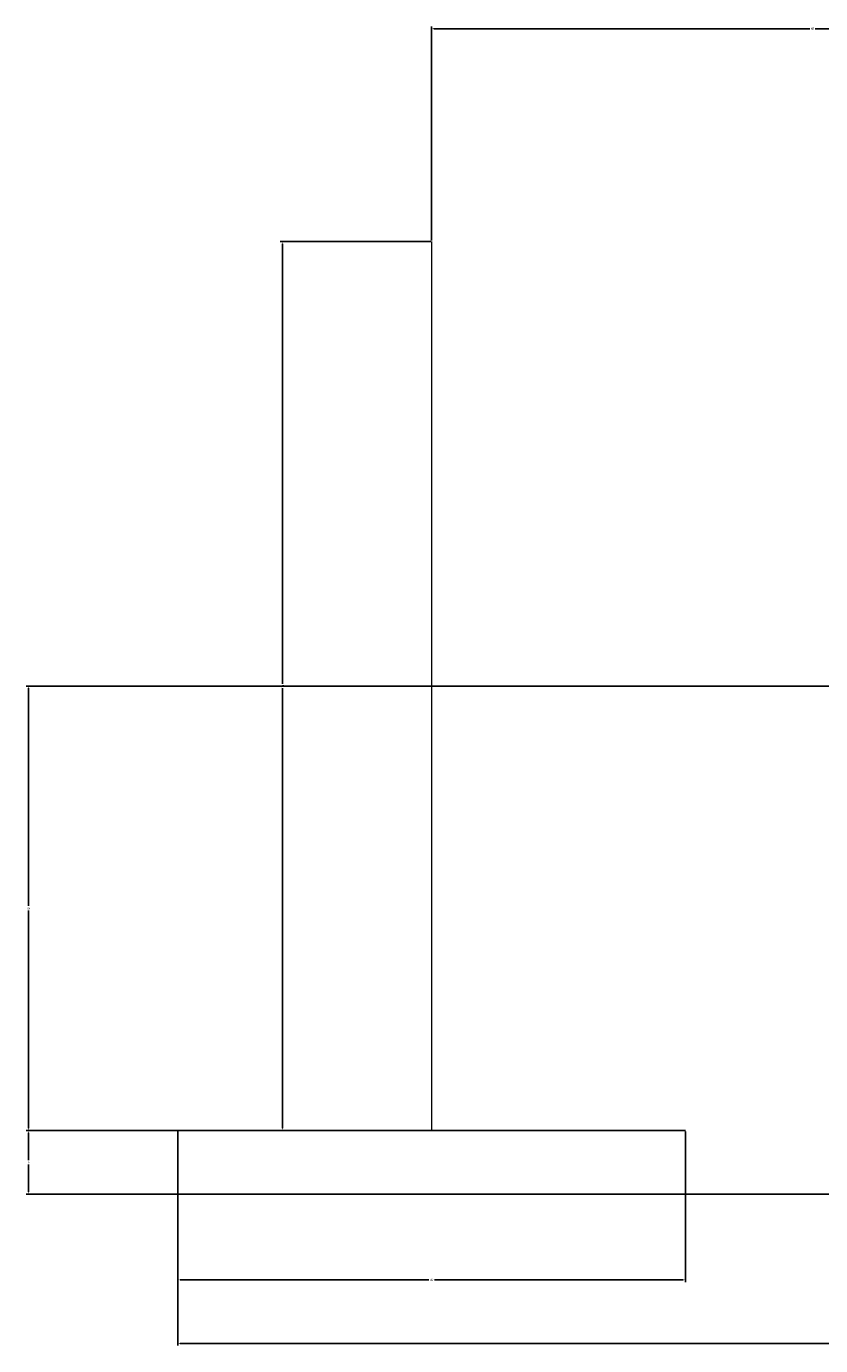
# Model space of a CAD drawing. Units: millimetres. Extents: x 3108 to 3332, y 1482 to 1586.
# Tile 1 of 5: x 3108 to 3171, y 1482 to 1586. Entities that reach past the tile are written whole.
import ezdxf

# ---------------------------------------------------------------- set-up
doc = ezdxf.new("R2010")
doc.units = ezdxf.units.MM
doc.layers.add('M-CONS', color=8, linetype='Continuous', lineweight=18)
doc.layers.add('M-DIMS', color=2, linetype='Continuous', lineweight=18)
doc.styles.get("Standard").update_dxf_attribs({"font": 'arial.ttf'})
doc.dimstyles.get("Standard").update_dxf_attribs({"dimtxt": 0.18, "dimasz": 0.18, "dimexe": 0.18, "dimexo": 0.0625, "dimgap": 0.09, "dimtad": 0, "dimtih": 1, "dimtoh": 1, "dimdec": 4, "dimzin": 0, "dimdsep": 46, "dimtxsty": 'Standard', "dimcen": 0.09, "dimadec": 0, "dimazin": 0, "dimtfac": 1, "dimtdec": 4, "dimtofl": 0, "dimtmove": 0, "dimatfit": 3, "dimfxl": 1, "dimtolj": 1, "dimtzin": 0, "dimarcsym": 0})

# ---------------------------------------------------------------- blocks, each defined once
blk = doc.blocks.new('*D1')
at = {"layer": 'Defpoints', "color": 0, "transparency": 16777216}
for p in [(3119.94, 1498.94), (3319.94, 1493.94), (3319.94, 1482.19)]:
    blk.add_point(p, dxfattribs=at)
at = {"layer": 'M-DIMS', "color": 0, "lineweight": -2, "transparency": 16777216}
for p, q in [((3119.94, 1498.88), (3119.94, 1482.01)), ((3319.94, 1493.88), (3319.94, 1482.01)), ((3120.12, 1482.19), (3219.65, 1482.19)), ((3319.76, 1482.19), (3220.23, 1482.19))]:
    blk.add_line(p, q, dxfattribs=at)
at = {"layer": 'M-DIMS', "color": 0, "transparency": 16777216}
for points in [[(3120.12, 1482.22), (3120.12, 1482.16), (3119.94, 1482.19)], [(3319.76, 1482.22), (3319.76, 1482.16), (3319.94, 1482.19)]]:
    blk.add_solid(points, dxfattribs=at)
at = {"layer": 'M-DIMS', "color": 0, "transparency": 16777216, "insert": (3219.94, 1482.19), "char_height": 0.18, "attachment_point": 5}
blk.add_mtext('\\A1;200', dxfattribs=at)
blk = doc.blocks.new('*D4')
at = {"layer": 'Defpoints', "color": 0, "transparency": 16777216}
for p in [(3119.94, 1498.94), (3159.94, 1498.94), (3119.94, 1487.19)]:
    blk.add_point(p, dxfattribs=at)
at = {"layer": 'M-DIMS', "color": 0, "lineweight": -2, "transparency": 16777216}
for p, q in [((3119.94, 1498.88), (3119.94, 1487.01)), ((3159.94, 1498.88), (3159.94, 1487.01)), ((3120.12, 1487.19), (3139.72, 1487.19)), ((3159.76, 1487.19), (3140.17, 1487.19))]:
    blk.add_line(p, q, dxfattribs=at)
at = {"layer": 'M-DIMS', "color": 0, "transparency": 16777216}
for points in [[(3120.12, 1487.22), (3120.12, 1487.16), (3119.94, 1487.19)], [(3159.76, 1487.22), (3159.76, 1487.16), (3159.94, 1487.19)]]:
    blk.add_solid(points, dxfattribs=at)
at = {"layer": 'M-DIMS', "color": 0, "transparency": 16777216, "insert": (3139.94, 1487.19), "char_height": 0.18, "attachment_point": 5}
blk.add_mtext('\\A1;40', dxfattribs=at)
blk = doc.blocks.new('*D5')
at = {"layer": 'Defpoints', "color": 0, "transparency": 16777216}
for p in [(3128.19, 1568.94), (3139.94, 1568.94), (3139.94, 1498.94)]:
    blk.add_point(p, dxfattribs=at)
at = {"layer": 'M-DIMS', "color": 0, "lineweight": -2, "transparency": 16777216}
for p, q in [((3139.88, 1568.94), (3128.01, 1568.94)), ((3128.19, 1568.76), (3128.19, 1534.12)), ((3128.19, 1499.12), (3128.19, 1533.76)), ((3139.88, 1498.94), (3128.01, 1498.94))]:
    blk.add_line(p, q, dxfattribs=at)
at = {"layer": 'M-DIMS', "color": 0, "transparency": 16777216}
for points in [[(3128.16, 1568.76), (3128.22, 1568.76), (3128.19, 1568.94)], [(3128.16, 1499.12), (3128.22, 1499.12), (3128.19, 1498.94)]]:
    blk.add_solid(points, dxfattribs=at)
at = {"layer": 'M-DIMS', "color": 0, "transparency": 16777216, "insert": (3128.19, 1533.94), "char_height": 0.18, "attachment_point": 5}
blk.add_mtext('\\A1;70', dxfattribs=at)
blk = doc.blocks.new('*D6')
at = {"layer": 'Defpoints', "color": 0, "transparency": 16777216}
for p in [(3199.94, 1585.69), (3139.94, 1568.94), (3199.94, 1533.94)]:
    blk.add_point(p, dxfattribs=at)
at = {"layer": 'M-DIMS', "color": 0, "lineweight": -2, "transparency": 16777216}
for p, q in [((3139.94, 1569.01), (3139.94, 1585.87)), ((3140.12, 1585.69), (3169.73, 1585.69)), ((3199.76, 1585.69), (3170.16, 1585.69)), ((3199.94, 1534.01), (3199.94, 1585.87))]:
    blk.add_line(p, q, dxfattribs=at)
at = {"layer": 'M-DIMS', "color": 0, "transparency": 16777216}
for points in [[(3140.12, 1585.72), (3140.12, 1585.66), (3139.94, 1585.69)], [(3199.76, 1585.72), (3199.76, 1585.66), (3199.94, 1585.69)]]:
    blk.add_solid(points, dxfattribs=at)
at = {"layer": 'M-DIMS', "color": 0, "transparency": 16777216, "insert": (3169.94, 1585.69), "char_height": 0.18, "attachment_point": 5}
blk.add_mtext('\\A1;60', dxfattribs=at)
blk = doc.blocks.new('*D9')
at = {"layer": 'Defpoints', "color": 0, "transparency": 16777216}
for p in [(3108.19, 1533.94), (3199.94, 1533.94), (3159.94, 1498.94)]:
    blk.add_point(p, dxfattribs=at)
at = {"layer": 'M-DIMS', "color": 0, "lineweight": -2, "transparency": 16777216}
for p, q in [((3199.88, 1533.94), (3108.01, 1533.94)), ((3108.19, 1533.76), (3108.19, 1516.63)), ((3108.19, 1499.12), (3108.19, 1516.26)), ((3159.88, 1498.94), (3108.01, 1498.94))]:
    blk.add_line(p, q, dxfattribs=at)
at = {"layer": 'M-DIMS', "color": 0, "transparency": 16777216}
for points in [[(3108.16, 1533.76), (3108.22, 1533.76), (3108.19, 1533.94)], [(3108.16, 1499.12), (3108.22, 1499.12), (3108.19, 1498.94)]]:
    blk.add_solid(points, dxfattribs=at)
at = {"layer": 'M-DIMS', "color": 0, "transparency": 16777216, "insert": (3108.19, 1516.44), "char_height": 0.18, "attachment_point": 5}
blk.add_mtext('\\A1;35', dxfattribs=at)
blk = doc.blocks.new('*D10')
at = {"layer": 'Defpoints', "color": 0, "transparency": 16777216}
for p in [(3119.94, 1498.94), (3108.19, 1493.94), (3319.94, 1493.94)]:
    blk.add_point(p, dxfattribs=at)
at = {"layer": 'M-DIMS', "color": 0, "lineweight": -2, "transparency": 16777216}
for p, q in [((3119.88, 1498.94), (3108.01, 1498.94)), ((3108.19, 1498.76), (3108.19, 1496.62)), ((3108.19, 1494.12), (3108.19, 1496.26)), ((3319.88, 1493.94), (3108.01, 1493.94))]:
    blk.add_line(p, q, dxfattribs=at)
at = {"layer": 'M-DIMS', "color": 0, "transparency": 16777216}
for points in [[(3108.16, 1498.76), (3108.22, 1498.76), (3108.19, 1498.94)], [(3108.16, 1494.12), (3108.22, 1494.12), (3108.19, 1493.94)]]:
    blk.add_solid(points, dxfattribs=at)
at = {"layer": 'M-DIMS', "color": 0, "transparency": 16777216, "insert": (3108.19, 1496.44), "char_height": 0.18, "attachment_point": 5}
blk.add_mtext('\\A1;5', dxfattribs=at)

msp = doc.modelspace()

# ---------------------------------------------------------------- linework, layer by layer
at = {"layer": 'M-CONS'}
msp.add_line((3139.9448, 1498.9431), (3139.9448, 1568.9431), dxfattribs=at)
at = {"layer": 'M-CONS', "extrusion": (0, -1, 0)}
msp.add_circle((3139.9448, 30, -1498.9431), 20, dxfattribs=at)

# ---------------------------------------------------------------- dimensions: what is measured, and where the dimension line sits
at = {"layer": 'M-DIMS'}
for base, p1, p2, picture, middle in [((3199.9448, 1585.6931), (3139.9448, 1568.9431), (3199.9448, 1533.9431), '*D6', (3169.9448, 1585.6931)), ((3319.9448, 1482.1931), (3119.9448, 1498.9431), (3319.9448, 1493.9431), '*D1', (3219.9448, 1482.1931))]:
    dim = msp.add_linear_dim(base=base, p1=p1, p2=p2, dimstyle='Standard', override={"dimdec": 0, "dimlfac": 1, "dimrnd": 0, "dimzin": 0, "dimdsep": 46, "dimlunit": 2}, dxfattribs=at)
    dim.commit()
    dim.dimension.update_dxf_attribs({"geometry": picture, "text_midpoint": middle})
for base, p1, p2, angle, picture, middle in [((3128.1948, 1568.9431), (3139.9448, 1498.9431), (3139.9448, 1568.9431), 90, '*D5', (3128.1948, 1533.9431)), ((3108.1948, 1533.9431), (3159.9448, 1498.9431), (3199.9448, 1533.9431), 90, '*D9', (3108.1948, 1516.4431)), ((3108.1948, 1493.9431), (3119.9448, 1498.9431), (3319.9448, 1493.9431), 90, '*D10', (3108.1948, 1496.4431)), ((3119.9448, 1487.1931), (3159.9448, 1498.9431), (3119.9448, 1498.9431), 180, '*D4', (3139.9448, 1487.1931))]:
    dim = msp.add_linear_dim(base=base, p1=p1, p2=p2, angle=angle, dimstyle='Standard', override={"dimdec": 0, "dimlfac": 1, "dimrnd": 0, "dimzin": 0, "dimdsep": 46, "dimlunit": 2}, dxfattribs=at)
    dim.commit()
    dim.dimension.update_dxf_attribs({"geometry": picture, "text_midpoint": middle})

doc.saveas('drawing.dxf')
